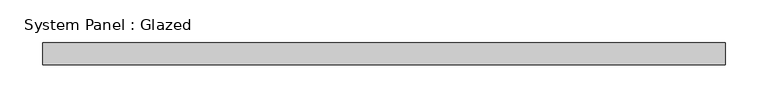
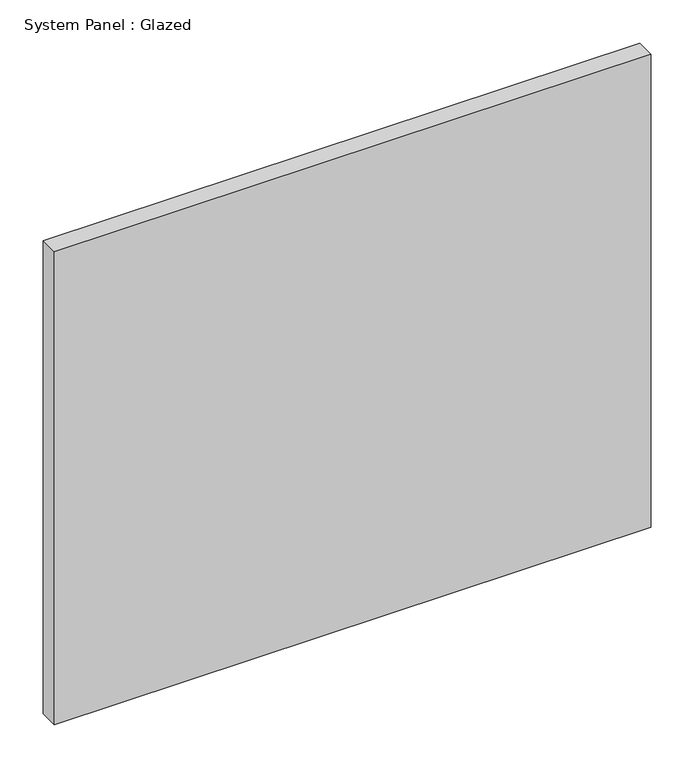
"""IFC4 building model written with IfcOpenShell, lengths in millimetres: plate geometry, System Panel : Glazed."""

from ifc_helpers import new_model, si_unit, origin, origin_with_axes, place, context, project, spatial, polyline, outline, extrude, source, transform, mapped, element, save


def system_panel_glazed_82a57ab2(model_context):
    return source(origin(), model_context, "Body", "SweptSolid", [
        extrude(outline(polyline([(397.9333333, 19.05), (-397.9333333, 19.05), (-397.9333333, 44.45), (397.9333333, 44.45), (397.9333333, 19.05)])), origin_with_axes(), (0.0, 0.0, 1.0), 666.75),
    ])


if __name__ == "__main__":
    model = new_model("IFC4")
    model_context = context("Model", 3, world=origin())
    ifc_project = project(units=[si_unit("LENGTHUNIT", "METRE", prefix="MILLI")], contexts=[model_context])
    site = spatial("IfcSite", under=ifc_project)
    building = spatial("IfcBuilding", under=site)
    placement = place(None, origin())
    system_panel_glazed_shape = system_panel_glazed_82a57ab2(model_context)
    element("IfcPlate", 1, ObjectType="System Panel : Glazed", at=placement, inside=building, context=model_context, shape_type="MappedRepresentation", body=[
        mapped(system_panel_glazed_shape, transform((0.0, 0.0, 0.0), x_axis=(1.0, 0.0, 0.0), y_axis=(0.0, 1.0, 0.0), z_axis=(0.0, 0.0, 1.0))),
    ])
    save(model, "model.ifc")

# Revit data of these elements
# Type "System Panel : Glazed"
#   Construction Type Id = "GSP4R"
#   Analytic Construction = "1/8 in Pilkington single glazing"
#   Visual Light Transmittance = 0.9
#   Solar Heat Gain Coefficient = 0.86
#   Heat Transfer Coefficient (U) = 1.18115 BTU/(h·ft²·°F)
# Element 1 (IfcPlate, "System Panel : Glazed")
#   Materials on its faces: "Glass"
# Materials
#   "Glass": class "Glass", colour RGB 0 128 192, transparency 0.75, Description = "Soda Lime Glass", Cost = 0
